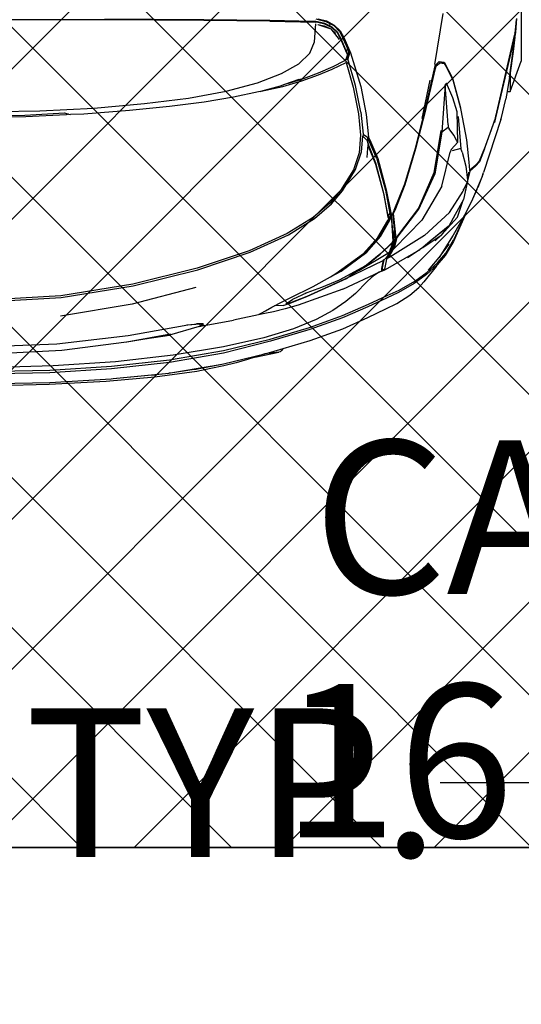
# Model space of a CAD drawing. Units: inches. Extents: x 2167 to 2589, y 1680 to 2489.
# Tile 5 of 38: x 2283 to 2307, y 1680 to 1727. Entities that reach past the tile are written whole.
import ezdxf

# ---------------------------------------------------------------- set-up
doc = ezdxf.new("R2010")
doc.units = ezdxf.units.IN
doc.header["$MEASUREMENT"] = 0
doc.layers.get('0').update_dxf_attribs({"color": 250})
for name, color, linetype, lineweight in [('A-ANNO-DIMS', 2, 'Continuous', 18), ('A-AREA-IDEN', 7, 'Continuous', 18), ('C-PRKG-VEHS', 8, 'Continuous', 13), ('C-PROP', 7, 'Continuous', 35), ('L-PVMT-PATT', 252, 'Continuous', 13)]:
    doc.layers.add(name, color=color, linetype=linetype, lineweight=lineweight)
doc.layers.add('Edges', color=250, linetype='Continuous')
doc.styles.get("Standard").update_dxf_attribs({"font": 'arial.ttf'})
doc.dimstyles.get("Standard").update_dxf_attribs({"dimtxt": 7, "dimasz": 0.18, "dimexe": 0.18, "dimexo": 0.0625, "dimgap": 0.09, "dimtad": 0, "dimtih": 1, "dimtoh": 1, "dimdec": 1, "dimzin": 0, "dimdsep": 46, "dimlunit": 3, "dimtxsty": 'Standard', "dimcen": 0.09, "dimadec": 0, "dimazin": 0, "dimtfac": 1, "dimtdec": 1, "dimtofl": 0, "dimtmove": 0, "dimatfit": 3, "dimfxl": 1, "dimtolj": 1, "dimtzin": 0, "dimarcsym": 0})

# ---------------------------------------------------------------- blocks, each defined once
blk = doc.blocks.new('Nissan Qashqai pl')
at = {"layer": 'Edges'}
for p, q in [((10.9577, 12.8101), (11.1283, 12.8101)), ((11.1783, 12.7921), (11.1283, 12.8101)), ((11.0576, 12.8026), (11.0798, 12.8008)), ((11.0768, 12.8008), (11.059, 12.8023)), ((11.0811, 12.8004), (11.0768, 12.8008)), ((11.0798, 12.8008), (11.0872, 12.7999)), ((11.0827, 12.8001), (11.0811, 12.8004)), ((11.0827, 12.8001), (11.0813, 12.7998)), ((11.0836, 12.8002), (11.0827, 12.8001)), ((11.0856, 12.7994), (11.0827, 12.8001)), ((11.0872, 12.7999), (11.0836, 12.8002)), ((11.0836, 12.8002), (11.0882, 12.7992)), ((11.2196, 12.7681), (11.0856, 12.7994)), ((11.0883, 12.7998), (11.0872, 12.7999)), ((11.0882, 12.7992), (11.2222, 12.7676)), ((11.0883, 12.7998), (11.1123, 12.797)), ((11.1147, 12.7965), (11.0883, 12.7998)), ((11.1123, 12.797), (11.1475, 12.7921)), ((11.1547, 12.791), (11.1147, 12.7965)), ((11.1475, 12.7921), (11.1525, 12.7914)), ((11.1475, 12.7921), (11.1783, 12.7921)), ((11.1525, 12.7914), (11.1547, 12.791)), ((11.1547, 12.791), (11.1783, 12.787)), ((11.1783, 12.787), (11.1783, 12.7921)), ((11.1783, 12.787), (11.1906, 12.7849)), ((11.1906, 12.7849), (11.1909, 12.7849)), ((11.193, 12.7845), (11.1909, 12.7849)), ((11.2215, 12.7775), (11.193, 12.7845)), ((11.2247, 12.7764), (11.2215, 12.7775)), ((11.2247, 12.7764), (11.3124, 12.7479)), ((11.2247, 12.767), (11.2163, 12.7689)), ((11.22, 12.768), (11.2196, 12.7681)), ((11.2247, 12.767), (11.22, 12.768)), ((11.2222, 12.7676), (11.2271, 12.7664)), ((11.2253, 12.7668), (11.2247, 12.767)), ((11.2304, 12.7649), (11.2253, 12.7668)), ((11.2253, 12.7668), (11.2271, 12.7664)), ((11.2271, 12.7664), (11.2296, 12.7658)), ((11.2271, 12.7664), (11.2277, 12.7662)), ((11.2277, 12.7662), (11.2296, 12.7658)), ((11.2732, 12.7496), (11.2277, 12.7662)), ((11.2704, 12.7504), (11.2304, 12.7649)), ((11.2702, 12.7507), (11.2704, 12.7504)), ((11.2704, 12.7506), (11.2707, 12.7503)), ((11.2707, 12.7503), (11.2704, 12.7504)), ((11.2719, 12.7498), (11.2707, 12.7503)), ((11.2934, 12.741), (11.2719, 12.7498)), ((11.2732, 12.7496), (11.2946, 12.7409)), ((11.3, 12.735), (11.2934, 12.741)), ((11.2946, 12.7409), (11.3018, 12.7346)), ((11.3161, 12.7467), (11.3124, 12.7479)), ((11.3161, 12.7467), (11.3376, 12.7381)), ((11.3192, 12.7454), (11.3566, 12.7294)), ((11.2956, 12.7234), (11.3085, 12.7247)), ((11.3081, 12.7253), (11.3, 12.735)), ((11.3018, 12.7346), (11.3103, 12.7249)), ((11.3086, 12.7247), (11.3081, 12.7253)), ((11.3081, 12.7253), (11.3087, 12.7247)), ((11.3085, 12.7247), (11.3086, 12.7247)), ((11.3086, 12.7247), (11.3087, 12.7247)), ((11.3087, 12.7247), (11.3103, 12.7249)), ((11.3103, 12.7249), (11.3103, 12.7249)), ((11.3103, 12.7249), (11.3106, 12.7249)), ((11.3106, 12.7249), (11.314, 12.7238)), ((11.3132, 12.7243), (11.3256, 12.7215)), ((11.3405, 12.7369), (11.3376, 12.7381)), ((11.3405, 12.7369), (11.3566, 12.7294)), ((11.3566, 12.7294), (11.3796, 12.7187)), ((11.156, 12.6966), (11.203, 12.7093)), ((11.1589, 12.6971), (11.2062, 12.7098)), ((11.203, 12.7093), (11.2091, 12.7103)), ((11.2062, 12.7098), (11.2091, 12.7103)), ((11.2091, 12.7103), (11.2583, 12.7196)), ((11.2199, 12.706), (11.2666, 12.7097)), ((11.2583, 12.7196), (11.2956, 12.7234)), ((11.2666, 12.7097), (11.2729, 12.7104)), ((11.2787, 12.7123), (11.2729, 12.7104)), ((11.2729, 12.7104), (11.2766, 12.6957)), ((11.2787, 12.7123), (11.3022, 12.7186)), ((11.3022, 12.7186), (11.3252, 12.7213)), ((11.317, 12.7227), (11.3119, 12.7236)), ((11.314, 12.7238), (11.317, 12.7227)), ((11.314, 12.7238), (11.3242, 12.7216)), ((11.3242, 12.7216), (11.317, 12.7227)), ((11.3198, 12.7211), (11.3252, 12.7213)), ((11.3242, 12.7216), (11.3256, 12.7215)), ((11.3252, 12.7213), (11.3283, 12.7214)), ((11.3256, 12.7215), (11.3283, 12.7214)), ((11.3283, 12.7214), (11.3297, 12.7206)), ((11.3297, 12.7206), (11.3446, 12.7173)), ((11.3297, 12.7206), (11.3302, 12.7203)), ((11.3302, 12.7203), (11.3446, 12.7173)), ((11.3302, 12.7203), (11.3394, 12.7152)), ((11.3394, 12.7152), (11.3434, 12.7138)), ((11.3394, 12.7152), (11.342, 12.7137)), ((11.379, 12.6915), (11.3434, 12.7138)), ((11.3446, 12.7173), (11.3571, 12.7146)), ((11.3583, 12.7142), (11.3571, 12.7146)), ((11.3571, 12.7146), (11.3821, 12.7008)), ((11.3583, 12.7142), (11.3821, 12.7008)), ((11.3864, 12.7044), (11.3583, 12.7142)), ((11.3796, 12.7187), (11.4164, 12.6974)), ((11.3796, 12.7187), (11.3807, 12.7182)), ((11.3807, 12.7182), (11.4267, 12.6979)), ((11.4228, 12.6989), (11.3807, 12.7182)), ((11.1298, 12.6823), (11.156, 12.6966)), ((11.1365, 12.6851), (11.1589, 12.6971)), ((11.189, 12.6968), (11.1644, 12.6862)), ((11.2121, 12.7043), (11.189, 12.6968)), ((11.2622, 12.7051), (11.2121, 12.7043)), ((11.2505, 12.6987), (11.2401, 12.6908)), ((11.2601, 12.7037), (11.2505, 12.6987)), ((11.2622, 12.7051), (11.2601, 12.7037)), ((11.2743, 12.6942), (11.2622, 12.7051)), ((11.2743, 12.6942), (11.2791, 12.6927)), ((11.335, 12.6786), (11.2791, 12.6927)), ((11.379, 12.6915), (11.417, 12.6499)), ((11.3821, 12.7008), (11.4014, 12.69)), ((11.4163, 12.6775), (11.3864, 12.7044)), ((11.4164, 12.6974), (11.4531, 12.6744)), ((11.4243, 12.6982), (11.4228, 12.6989)), ((11.4464, 12.6853), (11.4243, 12.6982)), ((11.4267, 12.6979), (11.4498, 12.6844)), ((11.1336, 12.667), (11.0492, 12.6807)), ((11.1285, 12.6745), (11.1298, 12.6823)), ((11.1306, 12.6812), (11.1293, 12.6736)), ((11.1306, 12.6752), (11.1319, 12.6827)), ((11.1319, 12.6827), (11.1306, 12.6812)), ((11.1347, 12.671), (11.1306, 12.6752)), ((11.1319, 12.6827), (11.1365, 12.6851)), ((11.1644, 12.6862), (11.1672, 12.6844)), ((11.2337, 12.6892), (11.1672, 12.6844)), ((11.1672, 12.6844), (11.2459, 12.6785)), ((11.2337, 12.6892), (11.2382, 12.6892)), ((11.2382, 12.6892), (11.2401, 12.6908)), ((11.2382, 12.6892), (11.2459, 12.6785)), ((11.2428, 12.6769), (11.3132, 12.6652)), ((11.2459, 12.6785), (11.3153, 12.6672)), ((11.335, 12.6786), (11.3915, 12.6453)), ((11.4014, 12.69), (11.4022, 12.6894)), ((11.4014, 12.69), (11.4265, 12.6594)), ((11.4022, 12.6894), (11.4163, 12.6775)), ((11.4022, 12.6894), (11.4265, 12.6594)), ((11.4366, 12.6471), (11.4163, 12.6775)), ((11.4163, 12.6775), (11.4259, 12.6674)), ((11.4531, 12.6744), (11.4314, 12.6911)), ((11.4624, 12.6717), (11.4464, 12.6853)), ((11.4498, 12.6844), (11.4662, 12.6706)), ((11.4681, 12.6691), (11.4498, 12.6844)), ((11.1293, 12.6736), (11.1285, 12.6745)), ((11.1353, 12.6677), (11.1293, 12.6736)), ((11.1366, 12.6691), (11.1347, 12.671)), ((11.1358, 12.6676), (11.1353, 12.6677)), ((11.1358, 12.6676), (11.1366, 12.6691)), ((11.148, 12.665), (11.1358, 12.6676)), ((11.1401, 12.6682), (11.1366, 12.6691)), ((11.2066, 12.6527), (11.1401, 12.6682)), ((11.2063, 12.6515), (11.148, 12.665)), ((11.2232, 12.6458), (11.1598, 12.6594)), ((11.3132, 12.6652), (11.3715, 12.6398)), ((11.3733, 12.6404), (11.3153, 12.6672)), ((11.4265, 12.6594), (11.4366, 12.6471)), ((11.4742, 12.6567), (11.4531, 12.6744)), ((11.4774, 12.6543), (11.4624, 12.6717)), ((11.4662, 12.6706), (11.4815, 12.6531)), ((11.4681, 12.6691), (11.4936, 12.6491)), ((11.272, 12.6349), (11.2063, 12.6515)), ((11.2728, 12.6357), (11.2066, 12.6527)), ((11.3915, 12.6453), (11.4381, 12.6002)), ((11.417, 12.6499), (11.4529, 12.5922)), ((11.4366, 12.6471), (11.4408, 12.6419)), ((11.4924, 12.6339), (11.4774, 12.6543)), ((11.4815, 12.6531), (11.4963, 12.6328)), ((11.4936, 12.6491), (11.5033, 12.6408)), ((11.3311, 12.6172), (11.272, 12.6349)), ((11.3323, 12.6178), (11.2728, 12.6357)), ((11.3715, 12.6398), (11.4177, 12.6052)), ((11.4203, 12.6044), (11.3733, 12.6404)), ((11.4408, 12.6419), (11.4411, 12.6414)), ((11.4411, 12.6414), (11.4411, 12.6414)), ((11.4414, 12.6409), (11.4411, 12.6414)), ((11.4414, 12.6409), (11.447, 12.6315)), ((11.4455, 12.6336), (11.4414, 12.6409)), ((11.447, 12.6315), (11.4455, 12.6336)), ((11.4455, 12.6336), (11.4462, 12.6324)), ((11.447, 12.6315), (11.4462, 12.6324)), ((11.4732, 12.585), (11.4462, 12.6324)), ((11.447, 12.6315), (11.447, 12.6314)), ((11.4536, 12.6215), (11.447, 12.6314)), ((11.5074, 12.608), (11.4924, 12.6339)), ((11.4964, 12.6326), (11.4963, 12.6328)), ((11.4964, 12.6326), (11.5113, 12.6069)), ((11.5158, 12.6256), (11.5033, 12.6408)), ((11.3751, 12.5999), (11.3311, 12.6172)), ((11.3747, 12.6011), (11.3323, 12.6178)), ((11.5295, 12.6041), (11.5158, 12.6256)), ((11.3411, 12.5863), (11.3795, 12.5939)), ((11.38, 12.5988), (11.3747, 12.6011)), ((11.3751, 12.5999), (11.3762, 12.5999)), ((11.3752, 12.5998), (11.3751, 12.5999)), ((11.3763, 12.5998), (11.3752, 12.5998)), ((11.3764, 12.5993), (11.3752, 12.5998)), ((11.3792, 12.5982), (11.3764, 12.5993)), ((11.3792, 12.5982), (11.3793, 12.5979)), ((11.3792, 12.5982), (11.3804, 12.5972)), ((11.3795, 12.5939), (11.3834, 12.5947)), ((11.3853, 12.5993), (11.38, 12.5988)), ((11.3804, 12.5972), (11.4082, 12.5998)), ((11.3827, 12.5953), (11.3804, 12.5972)), ((11.3804, 12.5926), (11.3841, 12.5933)), ((11.3811, 12.5958), (11.3808, 12.5961)), ((11.3834, 12.5947), (11.3827, 12.5953)), ((11.3846, 12.5953), (11.3829, 12.5952)), ((11.3829, 12.5952), (11.3849, 12.5951)), ((11.388, 12.591), (11.3829, 12.5952)), ((11.3834, 12.5947), (11.3841, 12.5933)), ((11.3846, 12.5953), (11.4248, 12.5976)), ((11.3846, 12.5953), (11.3846, 12.5953)), ((11.3851, 12.5951), (11.3846, 12.5953)), ((11.3846, 12.5953), (11.3849, 12.5951)), ((11.3849, 12.5951), (11.3851, 12.5951)), ((11.3882, 12.5923), (11.3849, 12.5951)), ((11.3851, 12.5951), (11.3867, 12.5949)), ((11.4171, 12.5766), (11.3851, 12.5951)), ((11.4212, 12.603), (11.3853, 12.5993)), ((11.3867, 12.5949), (11.3915, 12.5951)), ((11.3914, 12.5926), (11.3867, 12.5949)), ((11.3915, 12.5951), (11.4266, 12.5977)), ((11.409, 12.5999), (11.4082, 12.5998)), ((11.4164, 12.5998), (11.4082, 12.5998)), ((11.4152, 12.6004), (11.409, 12.5999)), ((11.409, 12.5999), (11.4163, 12.5999)), ((11.4173, 12.6006), (11.4152, 12.6004)), ((11.4163, 12.5999), (11.4152, 12.6004)), ((11.4163, 12.5999), (11.4186, 12.5999)), ((11.4164, 12.5998), (11.4163, 12.5999)), ((11.4181, 12.5998), (11.4164, 12.5998)), ((11.4169, 12.5996), (11.4164, 12.5998)), ((11.4252, 12.598), (11.4169, 12.5996)), ((11.4176, 12.6007), (11.4173, 12.6006)), ((11.418, 12.6006), (11.4173, 12.6006)), ((11.4215, 12.601), (11.4176, 12.6007)), ((11.418, 12.6006), (11.4176, 12.6007)), ((11.4177, 12.6052), (11.4193, 12.6042)), ((11.4204, 12.6002), (11.418, 12.6006)), ((11.4194, 12.6), (11.418, 12.6006)), ((11.4192, 12.6045), (11.4194, 12.6042)), ((11.4194, 12.6042), (11.4193, 12.6042)), ((11.4193, 12.6042), (11.4196, 12.604)), ((11.4194, 12.6042), (11.4196, 12.604)), ((11.4196, 12.6042), (11.4194, 12.6042)), ((11.4196, 12.604), (11.4201, 12.6036)), ((11.4198, 12.6041), (11.4201, 12.6036)), ((11.4201, 12.6036), (11.4212, 12.603)), ((11.4292, 12.6024), (11.4203, 12.6044)), ((11.4229, 12.6025), (11.4203, 12.6044)), ((11.4212, 12.603), (11.4215, 12.601)), ((11.4218, 12.6028), (11.4212, 12.603)), ((11.4215, 12.601), (11.4219, 12.6009)), ((11.4222, 12.6029), (11.4218, 12.6028)), ((11.4229, 12.6025), (11.4218, 12.6028)), ((11.4219, 12.6009), (11.4222, 12.6005)), ((11.4219, 12.6009), (11.4224, 12.6008)), ((11.4224, 12.6008), (11.4226, 12.6006)), ((11.4224, 12.6008), (11.423, 12.6006)), ((11.4315, 12.6002), (11.4229, 12.6025)), ((11.423, 12.6006), (11.4229, 12.6025)), ((11.44, 12.5959), (11.423, 12.6006)), ((11.4248, 12.5976), (11.4266, 12.5977)), ((11.4266, 12.5977), (11.4252, 12.598)), ((11.4266, 12.5977), (11.4268, 12.5977)), ((11.4268, 12.5977), (11.4296, 12.5954)), ((11.4268, 12.5977), (11.4278, 12.5977)), ((11.4303, 12.5956), (11.4278, 12.5977)), ((11.4278, 12.5977), (11.43, 12.5969)), ((11.4381, 12.6002), (11.4292, 12.6024)), ((11.4296, 12.5954), (11.4469, 12.5773)), ((11.4337, 12.5962), (11.43, 12.5969)), ((11.43, 12.5969), (11.4361, 12.5948)), ((11.4479, 12.5766), (11.4303, 12.5956)), ((11.4403, 12.5978), (11.4315, 12.6002)), ((11.4397, 12.5937), (11.4337, 12.5962)), ((11.4361, 12.5948), (11.4406, 12.5932)), ((11.4381, 12.6002), (11.4403, 12.5978)), ((11.4406, 12.5932), (11.4397, 12.5937)), ((11.4403, 12.5978), (11.44, 12.5959)), ((11.44, 12.5959), (11.4457, 12.5928)), ((11.4462, 12.5947), (11.4403, 12.5978)), ((11.452, 12.591), (11.4462, 12.5947)), ((11.5165, 12.5882), (11.5074, 12.608)), ((11.5113, 12.6068), (11.5113, 12.6069)), ((11.5113, 12.6068), (11.5206, 12.5869)), ((11.5384, 12.5859), (11.5295, 12.6041)), ((11.2895, 12.5724), (11.3411, 12.5863)), ((11.29, 12.5711), (11.3419, 12.585)), ((11.3474, 12.5827), (11.2972, 12.5692)), ((11.3493, 12.5828), (11.2993, 12.5695)), ((11.3419, 12.585), (11.3804, 12.5926)), ((11.3847, 12.5899), (11.3474, 12.5827)), ((11.3474, 12.5827), (11.3474, 12.5827)), ((11.3863, 12.5898), (11.3493, 12.5828)), ((11.3847, 12.5899), (11.3804, 12.5926)), ((11.3847, 12.5899), (11.3848, 12.5899)), ((11.388, 12.591), (11.3848, 12.5899)), ((11.3895, 12.5912), (11.3863, 12.5898)), ((11.3886, 12.5919), (11.3872, 12.5927)), ((11.3882, 12.5923), (11.3886, 12.5919)), ((11.3886, 12.5919), (11.3895, 12.5912)), ((11.3892, 12.5916), (11.3886, 12.5919)), ((11.3923, 12.5894), (11.3895, 12.5912)), ((11.4187, 12.5768), (11.3914, 12.5926)), ((11.4203, 12.5724), (11.3923, 12.5894)), ((11.4406, 12.5932), (11.4442, 12.592)), ((11.4442, 12.592), (11.4497, 12.589)), ((11.4462, 12.5893), (11.4442, 12.592)), ((11.4457, 12.5928), (11.4512, 12.5893)), ((11.475, 12.5409), (11.4462, 12.5893)), ((11.4469, 12.5773), (11.4659, 12.5539)), ((11.4497, 12.589), (11.4498, 12.5889)), ((11.4535, 12.5876), (11.4498, 12.5889)), ((11.4498, 12.5889), (11.4549, 12.5855)), ((11.4512, 12.5893), (11.4535, 12.5876)), ((11.4539, 12.5897), (11.452, 12.591)), ((11.4529, 12.5922), (11.4542, 12.5894)), ((11.4535, 12.5876), (11.4532, 12.5882)), ((11.4535, 12.5876), (11.4542, 12.5894)), ((11.4535, 12.5876), (11.4728, 12.5838)), ((11.4542, 12.5894), (11.4539, 12.5897)), ((11.4549, 12.5855), (11.4568, 12.5836)), ((11.4564, 12.5833), (11.4567, 12.5833)), ((11.4569, 12.583), (11.4565, 12.5831)), ((11.4568, 12.5836), (11.4571, 12.5833)), ((11.4571, 12.5833), (11.4573, 12.583)), ((11.4573, 12.583), (11.4578, 12.5822)), ((11.4704, 12.5803), (11.4573, 12.583)), ((11.4573, 12.5823), (11.4574, 12.5822)), ((11.4573, 12.5823), (11.4573, 12.5823)), ((11.4576, 12.5822), (11.4574, 12.5822)), ((11.4578, 12.5822), (11.4588, 12.5807)), ((11.4605, 12.5816), (11.4578, 12.5822)), ((11.4588, 12.5807), (11.4895, 12.5178)), ((11.4713, 12.5794), (11.4605, 12.5816)), ((11.4742, 12.5797), (11.4704, 12.5803)), ((11.4744, 12.5792), (11.4713, 12.5794)), ((11.4732, 12.585), (11.4728, 12.5838)), ((11.4728, 12.5838), (11.4742, 12.5797)), ((11.4728, 12.5838), (11.4746, 12.5796)), ((11.4758, 12.5791), (11.4732, 12.585)), ((11.4742, 12.5797), (11.4744, 12.5792)), ((11.4745, 12.5797), (11.4742, 12.5797)), ((11.4745, 12.5792), (11.4744, 12.5792)), ((11.4745, 12.5792), (11.4745, 12.5797)), ((11.4745, 12.5797), (11.4746, 12.5796)), ((11.4748, 12.5792), (11.4745, 12.5792)), ((11.4746, 12.5796), (11.4748, 12.5792)), ((11.4746, 12.5796), (11.4758, 12.5791)), ((11.4758, 12.5791), (11.4748, 12.5792)), ((11.4758, 12.5791), (11.4759, 12.579)), ((11.4759, 12.579), (11.4778, 12.5746)), ((11.4759, 12.579), (11.4771, 12.576)), ((11.5306, 12.5573), (11.5165, 12.5882)), ((11.5206, 12.5869), (11.5349, 12.5559)), ((11.5527, 12.5559), (11.5384, 12.5859)), ((11.29, 12.5711), (11.2541, 12.5557)), ((11.2586, 12.5591), (11.2895, 12.5724)), ((11.2972, 12.5692), (11.2677, 12.5575)), ((11.2993, 12.5695), (11.2705, 12.5579)), ((11.4433, 12.5543), (11.4171, 12.5766)), ((11.4447, 12.5545), (11.4187, 12.5768)), ((11.4467, 12.5488), (11.4203, 12.5724)), ((11.4654, 12.5548), (11.4479, 12.5766)), ((11.5057, 12.5145), (11.4771, 12.576)), ((11.4778, 12.5746), (11.4826, 12.5669)), ((11.4826, 12.5669), (11.4869, 12.5615)), ((11.4869, 12.5615), (11.4933, 12.555)), ((11.1144, 12.5271), (11.1702, 12.5444)), ((11.1702, 12.5444), (11.2166, 12.5534)), ((11.2127, 12.5443), (11.2488, 12.548)), ((11.2166, 12.5534), (11.2538, 12.5571)), ((11.2488, 12.548), (11.2541, 12.5557)), ((11.2488, 12.548), (11.2524, 12.5477)), ((11.2599, 12.5552), (11.2524, 12.5477)), ((11.2785, 12.5455), (11.2524, 12.5477)), ((11.2538, 12.5571), (11.2586, 12.5591)), ((11.2541, 12.5557), (11.2599, 12.5552)), ((11.2677, 12.5575), (11.2599, 12.5552)), ((11.265, 12.5563), (11.2599, 12.5552)), ((11.2705, 12.5579), (11.265, 12.5563)), ((11.265, 12.5563), (11.2724, 12.5557)), ((11.2724, 12.5557), (11.2874, 12.5544)), ((11.3076, 12.5358), (11.2785, 12.5455)), ((11.4745, 12.5116), (11.4433, 12.5543)), ((11.4758, 12.5118), (11.4447, 12.5545)), ((11.4801, 12.503), (11.4467, 12.5488)), ((11.4633, 12.5594), (11.4897, 12.5108)), ((11.4654, 12.5548), (11.4659, 12.5539)), ((11.4659, 12.5539), (11.4674, 12.5512)), ((11.4675, 12.551), (11.4674, 12.5512)), ((11.4675, 12.551), (11.4703, 12.546)), ((11.4703, 12.546), (11.4704, 12.5458)), ((11.4704, 12.5458), (11.4909, 12.5085)), ((11.4704, 12.5458), (11.4897, 12.5108)), ((11.5131, 12.5356), (11.4933, 12.555)), ((11.5496, 12.5141), (11.5306, 12.5573)), ((11.5349, 12.5559), (11.5535, 12.5139)), ((11.5716, 12.5145), (11.5527, 12.5559)), ((11.1683, 12.5354), (11.1244, 12.5227)), ((11.1302, 12.52), (11.1712, 12.5317)), ((11.2127, 12.5443), (11.1683, 12.5354)), ((11.1712, 12.5317), (11.2152, 12.5404)), ((11.2152, 12.5404), (11.2509, 12.5439)), ((11.2509, 12.5439), (11.28, 12.5414)), ((11.28, 12.5414), (11.3082, 12.532)), ((11.3428, 12.5139), (11.3076, 12.5358)), ((11.3082, 12.532), (11.3425, 12.5106)), ((11.475, 12.5409), (11.4828, 12.5276)), ((11.5131, 12.5356), (11.5265, 12.5194)), ((11.0779, 12.5103), (11.0902, 12.5166)), ((11.0787, 12.5092), (11.0908, 12.5153)), ((11.0902, 12.5166), (11.1144, 12.5271)), ((11.0908, 12.5153), (11.107, 12.5224)), ((11.1138, 12.5213), (11.0912, 12.5117)), ((11.1149, 12.5212), (11.0917, 12.5114)), ((11.107, 12.5224), (11.1116, 12.5243)), ((11.1138, 12.5213), (11.107, 12.5224)), ((11.1116, 12.5243), (11.1147, 12.5257)), ((11.1244, 12.5227), (11.1116, 12.5243)), ((11.1139, 12.5213), (11.1138, 12.5213)), ((11.1164, 12.5224), (11.1139, 12.5213)), ((11.1147, 12.5257), (11.1244, 12.5227)), ((11.1172, 12.5222), (11.1149, 12.5212)), ((11.1164, 12.5224), (11.1174, 12.5223)), ((11.1173, 12.5222), (11.1172, 12.5222)), ((11.1174, 12.5223), (11.1173, 12.5222)), ((11.12, 12.5215), (11.1174, 12.5223)), ((11.1246, 12.5199), (11.12, 12.5215)), ((11.1259, 12.5194), (11.1244, 12.5227)), ((11.1244, 12.5227), (11.126, 12.5194)), ((11.1259, 12.5194), (11.1246, 12.5199)), ((11.126, 12.5193), (11.1247, 12.5197)), ((11.126, 12.5193), (11.1248, 12.5195)), ((11.1251, 12.5189), (11.126, 12.5193)), ((11.126, 12.5193), (11.1259, 12.5194)), ((11.126, 12.5194), (11.1259, 12.5194)), ((11.126, 12.5194), (11.1261, 12.5193)), ((11.1264, 12.5192), (11.126, 12.5194)), ((11.1263, 12.5186), (11.126, 12.5193)), ((11.1261, 12.5193), (11.126, 12.5193)), ((11.1261, 12.5193), (11.1263, 12.5188)), ((11.1264, 12.5192), (11.1261, 12.5193)), ((11.1277, 12.5167), (11.1264, 12.5192)), ((11.1369, 12.4986), (11.1277, 12.5167)), ((11.1412, 12.4969), (11.1302, 12.52)), ((11.3645, 12.4958), (11.3428, 12.5139)), ((11.4852, 12.494), (11.4758, 12.5118)), ((11.488, 12.5208), (11.4828, 12.5276)), ((11.5179, 12.4551), (11.488, 12.5208)), ((11.4898, 12.5172), (11.4895, 12.5178)), ((11.4898, 12.5172), (11.49, 12.5167)), ((11.49, 12.5167), (11.5179, 12.4551)), ((11.5057, 12.5145), (11.5325, 12.4404)), ((11.5265, 12.5194), (11.541, 12.4982)), ((11.5691, 12.4592), (11.5496, 12.5141)), ((11.5535, 12.5139), (11.5726, 12.46)), ((11.5908, 12.4606), (11.5716, 12.5145)), ((11.0614, 12.4872), (11.0682, 12.5004)), ((11.0658, 12.4932), (11.0692, 12.4996)), ((11.0727, 12.4966), (11.0669, 12.4849)), ((11.0682, 12.5004), (11.0779, 12.5103)), ((11.0692, 12.4996), (11.0787, 12.5092)), ((11.0718, 12.4967), (11.0698, 12.4925)), ((11.0802, 12.5057), (11.0718, 12.4967)), ((11.0809, 12.5056), (11.0727, 12.4966)), ((11.0747, 12.4944), (11.092, 12.5087)), ((11.0747, 12.4944), (11.0821, 12.5029)), ((11.0912, 12.5117), (11.0802, 12.5057)), ((11.0917, 12.5114), (11.0809, 12.5056)), ((11.1475, 12.4741), (11.1369, 12.4986)), ((11.1505, 12.4742), (11.1412, 12.4969)), ((11.3425, 12.5106), (11.3635, 12.4929)), ((11.3888, 12.4678), (11.3645, 12.4958)), ((11.4788, 12.5052), (11.4745, 12.5116)), ((11.4801, 12.503), (11.4788, 12.5052)), ((11.4852, 12.494), (11.4801, 12.503)), ((11.4897, 12.5108), (11.4909, 12.5085)), ((11.4909, 12.5085), (11.5028, 12.4792)), ((11.541, 12.4982), (11.5562, 12.4701)), ((11.0581, 12.4738), (11.0614, 12.4872)), ((11.0582, 12.47), (11.0624, 12.4866)), ((11.0624, 12.4866), (11.0658, 12.4932)), ((11.0659, 12.4848), (11.063, 12.4728)), ((11.0669, 12.4849), (11.0641, 12.4733)), ((11.0658, 12.4932), (11.0698, 12.4925)), ((11.0698, 12.4925), (11.0659, 12.4848)), ((11.0671, 12.4731), (11.0747, 12.4944)), ((11.0671, 12.4731), (11.0696, 12.4836)), ((11.0696, 12.4836), (11.0747, 12.4944)), ((11.3635, 12.4929), (11.3872, 12.4654)), ((11.5013, 12.4651), (11.4852, 12.494)), ((11.5028, 12.4792), (11.5118, 12.4548)), ((11.0621, 12.4657), (11.0607, 12.3933)), ((11.0618, 12.3933), (11.0632, 12.47)), ((11.0622, 12.4697), (11.0621, 12.4657)), ((11.063, 12.4728), (11.0622, 12.4697)), ((11.0641, 12.4733), (11.0632, 12.47)), ((11.0962, 12.4675), (11.0662, 12.4698)), ((11.1148, 12.4598), (11.0962, 12.4675)), ((11.1577, 12.4465), (11.1475, 12.4741)), ((11.1605, 12.4465), (11.1505, 12.4742)), ((11.3872, 12.4654), (11.4138, 12.4223)), ((11.4159, 12.4242), (11.3888, 12.4678)), ((11.5202, 12.427), (11.5013, 12.4651)), ((11.5562, 12.4701), (11.5715, 12.4326)), ((11.1323, 12.4415), (11.1148, 12.4598)), ((11.1699, 12.4153), (11.1605, 12.4465)), ((11.5118, 12.4548), (11.523, 12.4311)), ((11.5118, 12.4548), (11.513, 12.4514)), ((11.5292, 12.4272), (11.5179, 12.4551)), ((11.5179, 12.4551), (11.5285, 12.4279)), ((11.5884, 12.3943), (11.5691, 12.4592)), ((11.5726, 12.46), (11.5922, 12.3947)), ((11.6042, 12.4156), (11.5908, 12.4606)), ((11.1487, 12.4126), (11.1323, 12.4415)), ((11.1643, 12.425), (11.1576, 12.4459)), ((11.1643, 12.425), (11.1577, 12.4465)), ((11.1582, 12.4416), (11.1668, 12.4177)), ((11.1583, 12.4423), (11.1643, 12.425)), ((11.5301, 12.4198), (11.523, 12.4311)), ((11.5325, 12.4404), (11.5386, 12.4187)), ((11.5715, 12.4326), (11.5866, 12.3835)), ((11.1643, 12.425), (11.1668, 12.4177)), ((11.1668, 12.4177), (11.1694, 12.4104)), ((11.178, 12.379), (11.1699, 12.4153)), ((11.4138, 12.4223), (11.4422, 12.3594)), ((11.4445, 12.3608), (11.4159, 12.4242)), ((11.5283, 12.4109), (11.5202, 12.427)), ((11.5285, 12.4279), (11.5302, 12.4209)), ((11.5331, 12.4157), (11.5292, 12.4272)), ((11.5302, 12.4209), (11.5301, 12.4198)), ((11.5331, 12.4157), (11.5335, 12.401)), ((11.5386, 12.4187), (11.5434, 12.3997)), ((11.6042, 12.4156), (11.6077, 12.4125)), ((11.6103, 12.395), (11.6042, 12.4156)), ((11.164, 12.373), (11.1487, 12.4126)), ((11.1694, 12.4104), (11.1781, 12.3782)), ((11.5334, 12.4014), (11.5283, 12.4109)), ((11.5326, 12.4045), (11.5333, 12.4019)), ((11.5333, 12.4019), (11.5334, 12.4014)), ((11.5335, 12.401), (11.5334, 12.4014)), ((11.5357, 12.3968), (11.5335, 12.401)), ((11.5434, 12.3997), (11.5461, 12.3854)), ((11.6077, 12.4125), (11.6094, 12.4107)), ((11.6094, 12.4107), (11.6101, 12.4085)), ((11.6101, 12.4085), (11.6127, 12.3852)), ((11.6185, 12.3689), (11.6101, 12.4085)), ((11.0607, 12.3933), (11.0595, 12.2842)), ((11.0618, 12.3933), (11.0606, 12.2841)), ((11.5416, 12.3863), (11.5357, 12.3968)), ((11.5455, 12.3793), (11.5416, 12.3863)), ((11.5461, 12.3854), (11.5467, 12.3822)), ((11.5467, 12.3822), (11.5571, 12.3331)), ((11.5866, 12.3835), (11.6016, 12.3166)), ((11.6076, 12.3166), (11.5884, 12.3943)), ((11.5922, 12.3947), (11.6118, 12.3165)), ((11.6127, 12.3852), (11.6103, 12.395)), ((11.6127, 12.3852), (11.6174, 12.3722)), ((11.6297, 12.3166), (11.6127, 12.3852)), ((11.1776, 12.3211), (11.164, 12.373)), ((11.1781, 12.3782), (11.178, 12.379)), ((11.1781, 12.3782), (11.1791, 12.3746)), ((11.1791, 12.3746), (11.1877, 12.333)), ((11.5472, 12.3757), (11.5455, 12.3793)), ((11.6174, 12.3722), (11.6185, 12.3689)), ((11.6185, 12.3689), (11.6224, 12.3567)), ((11.4422, 12.3594), (11.4712, 12.2729)), ((11.4738, 12.274), (11.4445, 12.3608)), ((11.6224, 12.3567), (11.6277, 12.3379)), ((11.1877, 12.333), (11.1958, 12.2844)), ((11.5668, 12.2816), (11.5571, 12.3331)), ((11.6277, 12.3379), (11.6328, 12.3174)), ((11.1891, 12.2586), (11.1776, 12.3211)), ((11.6016, 12.3166), (11.615, 12.2333)), ((11.6229, 12.2274), (11.6076, 12.3166)), ((11.6118, 12.3165), (11.6272, 12.2272)), ((11.6301, 12.3141), (11.6297, 12.3166)), ((11.6328, 12.3174), (11.6375, 12.2956)), ((11.6377, 12.2734), (11.6301, 12.3141)), ((11.6332, 12.2951), (11.6301, 12.3141)), ((11.0595, 12.2842), (11.0586, 12.1198)), ((11.0606, 12.2841), (11.0597, 12.1196)), ((11.1958, 12.2844), (11.2033, 12.2269)), ((11.566, 12.2846), (11.5668, 12.2816)), ((11.6334, 12.2946), (11.6332, 12.2951)), ((11.6443, 12.2288), (11.6334, 12.2946)), ((11.6375, 12.2956), (11.6422, 12.2725)), ((11.4712, 12.2729), (11.4976, 12.1662)), ((11.5005, 12.167), (11.4738, 12.274)), ((11.5033, 12.271), (11.5307, 12.165)), ((11.5626, 12.2771), (11.5627, 12.2817)), ((11.5627, 12.2746), (11.5626, 12.2771)), ((11.5626, 12.2745), (11.5627, 12.2746)), ((11.5627, 12.2817), (11.5634, 12.2829)), ((11.5627, 12.2817), (11.5633, 12.2814)), ((11.5628, 12.2721), (11.5627, 12.2746)), ((11.5632, 12.2783), (11.5633, 12.2814)), ((11.5636, 12.2706), (11.5632, 12.2783)), ((11.5633, 12.2814), (11.5634, 12.2829)), ((11.5633, 12.2814), (11.5661, 12.2803)), ((11.5634, 12.2829), (11.5668, 12.2816)), ((11.565, 12.2577), (11.5636, 12.2706)), ((11.5639, 12.2809), (11.5637, 12.2764)), ((11.5637, 12.2763), (11.5637, 12.2764)), ((11.5637, 12.2764), (11.5638, 12.2762)), ((11.5638, 12.2762), (11.5641, 12.2688)), ((11.5643, 12.2808), (11.5639, 12.2809)), ((11.5641, 12.2688), (11.5656, 12.2559)), ((11.5642, 12.2771), (11.5646, 12.2778)), ((11.566, 12.2801), (11.5643, 12.2808)), ((11.5647, 12.278), (11.5649, 12.2783)), ((11.566, 12.2801), (11.5661, 12.2803)), ((11.5662, 12.28), (11.566, 12.2801)), ((11.5661, 12.2803), (11.5662, 12.28)), ((11.5662, 12.28), (11.5661, 12.2803)), ((11.5669, 12.2797), (11.5661, 12.2803)), ((11.5669, 12.2797), (11.5662, 12.28)), ((11.5662, 12.28), (11.5662, 12.28)), ((11.5667, 12.2813), (11.567, 12.2796)), ((11.5668, 12.2816), (11.5672, 12.2796)), ((11.567, 12.2796), (11.5669, 12.2797)), ((11.5672, 12.2796), (11.567, 12.2796)), ((11.5678, 12.2766), (11.5672, 12.2796)), ((11.5673, 12.2784), (11.5677, 12.2767)), ((11.5678, 12.2766), (11.5818, 12.227)), ((11.5682, 12.2743), (11.5682, 12.2742)), ((11.5683, 12.2739), (11.5683, 12.2739)), ((11.5683, 12.2738), (11.5683, 12.2737)), ((11.6378, 12.2728), (11.6377, 12.2734)), ((11.6381, 12.2716), (11.6378, 12.2728)), ((11.639, 12.2645), (11.6378, 12.2728)), ((11.639, 12.2645), (11.6381, 12.2716)), ((11.6422, 12.2725), (11.6514, 12.2026)), ((11.1984, 12.1855), (11.1891, 12.2586)), ((11.5685, 12.2359), (11.565, 12.2577)), ((11.6443, 12.2288), (11.639, 12.2645)), ((11.5823, 12.1589), (11.5685, 12.2359)), ((11.2033, 12.2269), (11.21, 12.1607)), ((11.593, 12.1566), (11.58, 12.2288)), ((11.5883, 12.186), (11.5816, 12.2272)), ((11.5883, 12.186), (11.5818, 12.227)), ((11.615, 12.2333), (11.626, 12.1375)), ((11.6333, 12.131), (11.6229, 12.2274)), ((11.6272, 12.2272), (11.6377, 12.1308)), ((11.6446, 12.2271), (11.6443, 12.2288)), ((11.6448, 12.2258), (11.6446, 12.2271)), ((11.6474, 12.2042), (11.6448, 12.2258)), ((11.6539, 12.1338), (11.6448, 12.2258)), ((11.6474, 12.2038), (11.6474, 12.2042)), ((11.6475, 12.2032), (11.6474, 12.2038)), ((11.648, 12.198), (11.6475, 12.2032)), ((11.6514, 12.2026), (11.6589, 12.1222)), ((11.2057, 12.1019), (11.1984, 12.1855)), ((11.593, 12.1566), (11.5883, 12.186)), ((11.6539, 12.1338), (11.648, 12.198)), ((11.21, 12.1607), (11.2159, 12.085)), ((11.4976, 12.1662), (11.5166, 12.0471)), ((11.5196, 12.0475), (11.5005, 12.167)), ((11.5307, 12.165), (11.5504, 12.0466)), ((11.5963, 12.0406), (11.5823, 12.1589)), ((11.5932, 12.1556), (11.593, 12.1566)), ((11.6067, 12.0489), (11.5932, 12.1556)), ((11.626, 12.1375), (11.6329, 12.0344)), ((11.6399, 12.029), (11.6333, 12.131)), ((11.6377, 12.1308), (11.6444, 12.0289)), ((11.6543, 12.1306), (11.6539, 12.1338)), ((11.6604, 12.0287), (11.6543, 12.1306)), ((11.6589, 12.1222), (11.6635, 12.0274)), ((11.0597, 12.1196), (11.0594, 11.9221)), ((11.2101, 12.012), (11.2057, 12.1019)), ((11.2159, 12.085), (11.2166, 12.063)), ((11.2139, 12.0528), (11.2158, 12.0599)), ((11.2158, 12.0602), (11.2166, 12.063)), ((11.2158, 12.0602), (11.2168, 12.056)), ((11.2158, 12.0599), (11.2158, 12.0602)), ((11.2158, 12.0599), (11.2168, 12.056)), ((11.2168, 12.056), (11.2204, 11.989)), ((11.2174, 11.9874), (11.2139, 12.0528)), ((11.5166, 12.0471), (11.5239, 11.9221)), ((11.527, 11.9221), (11.5196, 12.0475)), ((11.6005, 11.9335), (11.5963, 12.0406)), ((11.6133, 11.9221), (11.6067, 12.0489)), ((11.6329, 12.0344), (11.6363, 11.9221)), ((11.6421, 11.9221), (11.6399, 12.029)), ((11.6444, 12.0289), (11.6465, 11.9221)), ((11.6623, 11.9221), (11.6604, 12.0287)), ((11.6635, 12.0274), (11.6663, 11.9221)), ((11.2116, 11.9221), (11.2101, 12.012)), ((11.218, 11.9221), (11.2174, 11.9874)), ((11.2204, 11.989), (11.2211, 11.9221))]:
    blk.add_line(p, q, dxfattribs=at)
blk = doc.blocks.new('car')
blk.add_blockref('Nissan Qashqai pl', (-9.7433, -11.9151))
blk = doc.blocks.new('carr')
blk.add_blockref('car', (0.5124, -0.007))
blk = doc.blocks.new('*D46')
at = {"layer": 'A-ANNO-DIMS', "color": 0, "lineweight": -2, "transparency": 16777216}
for p, q in [((2251.218, 1709.362), (2251.218, 1690.565)), ((2312.254, 1709.362), (2312.254, 1690.565)), ((2251.398, 1690.745), (2260.312, 1690.745)), ((2312.074, 1690.745), (2303.16, 1690.745))]:
    blk.add_line(p, q, dxfattribs=at)
at = {"layer": 'A-ANNO-DIMS', "color": 0, "transparency": 16777216}
for points in [[(2251.398, 1690.775), (2251.398, 1690.715), (2251.218, 1690.745)], [(2312.074, 1690.775), (2312.074, 1690.715), (2312.254, 1690.745)]]:
    blk.add_solid(points, dxfattribs=at)
at = {"layer": 'Defpoints', "color": 0, "transparency": 16777216}
for p in [(2251.218, 1709.425), (2312.254, 1709.425), (2312.254, 1690.745)]:
    blk.add_point(p, dxfattribs=at)
at = {"layer": 'A-ANNO-DIMS', "color": 0, "transparency": 16777216, "insert": (2281.736, 1690.745), "char_height": 7, "attachment_point": 5}
blk.add_mtext('\\A1;5\'-1" TYP.', dxfattribs=at)

msp = doc.modelspace()

# ---------------------------------------------------------------- hatches: boundary and pattern name
at = {"layer": 'L-PVMT-PATT'}
h = msp.add_hatch(dxfattribs=at)
h.set_pattern_fill('ANSI37', color=256, scale=40)
h.paths.add_polyline_path([(2417.548, 1783.695), (2417.548, 1846.042), (2239.361, 1846.042), (2239.361, 1687.695), (2369.843, 1687.695), (2369.843, 1696.695), (2375.607, 1696.695), (2416.107, 1696.695), (2417.548, 1696.695)])

# ---------------------------------------------------------------- linework, layer by layer
at = {"layer": 'C-PROP'}
msp.add_line((2575.048, 1687.695), (2215.048, 1687.695), dxfattribs=at)

# ---------------------------------------------------------------- block references
at = {"layer": 'C-PRKG-VEHS', "xscale": 28.42784210623918, "yscale": 28.42784210623918, "zscale": 28.42784210623918, "rotation": 270}
msp.add_blockref('carr', (2281.736, 1778.659), dxfattribs=at)

# ---------------------------------------------------------------- texts
at = {"layer": 'A-AREA-IDEN'}
for s, height, p in [('CAR PORCH', 7.2272, (2297.172, 1699.634)), ('16\'0" X 16\'0"', 7.22716, (2295.694, 1688.165))]:
    msp.add_text(s, height=height, dxfattribs=at).set_placement(p)

# ---------------------------------------------------------------- dimensions: what is measured, and where the dimension line sits
at = {"layer": 'A-ANNO-DIMS'}
dim = msp.add_linear_dim(base=(2312.254, 1690.745), p1=(2251.218, 1709.425), p2=(2312.254, 1709.425), text='<> TYP.', dimstyle='Standard', override={"dimdec": 1, "dimlfac": 1, "dimrnd": 0, "dimzin": 1, "dimdsep": 46, "dimlunit": 4, "dimfrac": 2}, dxfattribs=at)
dim.commit()
dim.dimension.update_dxf_attribs({"geometry": '*D46', "text_midpoint": (2281.736, 1690.745)})

doc.saveas('drawing.dxf')
